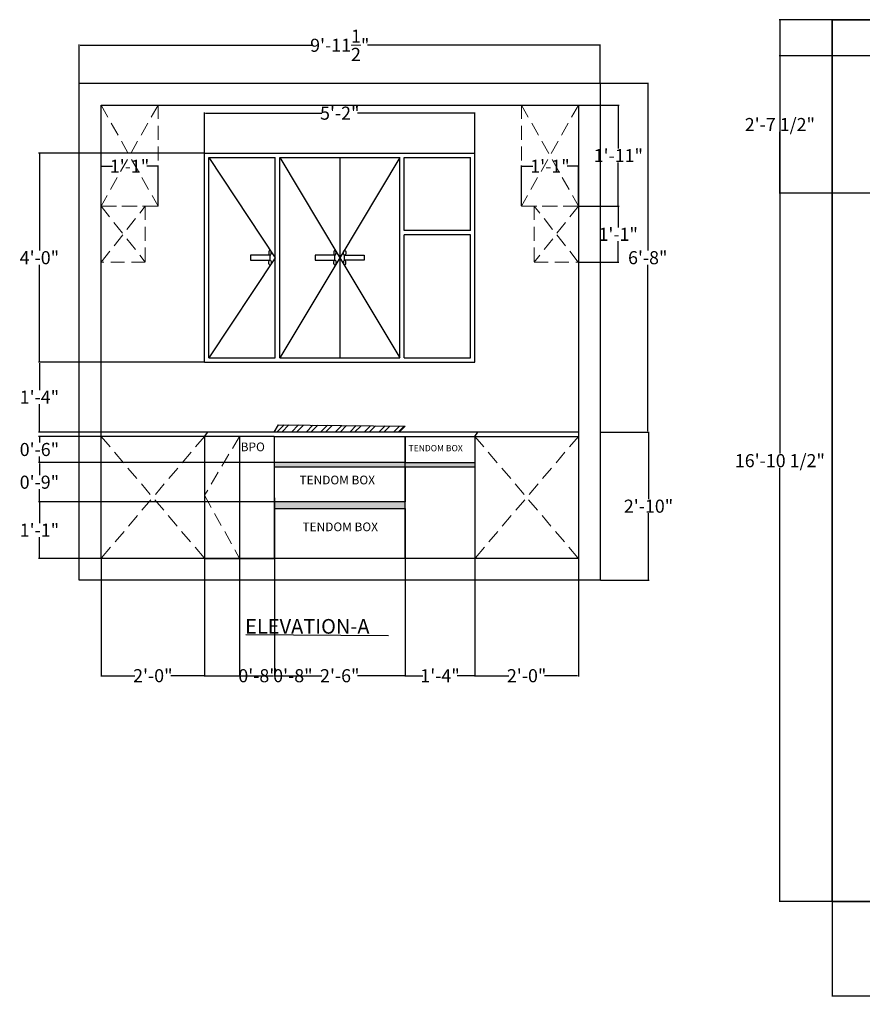
# Model space of a CAD drawing. Units: inches. Extents: x 1686244 to 1686928, y 1936095 to 1936489.
# Tile 1 of 11: x 1686285 to 1686478, y 1936095 to 1936321. Entities that reach past the tile are written whole.
import ezdxf

# ---------------------------------------------------------------- set-up
doc = ezdxf.new("R2010")
doc.units = ezdxf.units.IN
doc.header["$MEASUREMENT"] = 0
doc.linetypes.add('DASHED', pattern=[19.05, 12.7, -6.35])
for name, color, linetype, lineweight in [('A-ANNO-DIMS', 240, 'Continuous', 18), ('A-ANNO-TEXT', 7, 'Continuous', 18), ('A-CASE', 7, 'Continuous', 35), ('A-CASE-SWNG', 1, 'DASHED', 18), ('A-ELEV', 7, 'Continuous', 25), ('A-ELEV-PATT', 72, 'Continuous', 13)]:
    doc.layers.add(name, color=color, linetype=linetype, lineweight=lineweight)
doc.styles.get("Standard").update_dxf_attribs({"font": 'arial.ttf'})
doc.dimstyles.get("Standard").update_dxf_attribs({"dimtxt": 3, "dimasz": 0.18, "dimexe": 0.18, "dimexo": 0.0625, "dimgap": 0.09, "dimtad": 0, "dimtih": 1, "dimtoh": 1, "dimzin": 0, "dimdsep": 46, "dimlunit": 4, "dimtxsty": 'Standard', "dimcen": 0.09, "dimadec": 0, "dimazin": 0, "dimtfac": 1, "dimtofl": 0, "dimtmove": 0, "dimatfit": 3, "dimfxl": 1, "dimtolj": 1, "dimtzin": 0, "dimarcsym": 0})

# ---------------------------------------------------------------- blocks, each defined once
blk = doc.blocks.new('*D37')
at = {"layer": 'A-ANNO-DIMS', "color": 0, "lineweight": -2, "transparency": 16777216}
for p, q in [((1686298.55, 1936306.63), (1686298.55, 1936315.47)), ((1686298.73, 1936315.29), (1686351.96, 1936315.29)), ((1686417.87, 1936315.29), (1686364.63, 1936315.29)), ((1686418.05, 1936306.63), (1686418.05, 1936315.47))]:
    blk.add_line(p, q, dxfattribs=at)
at = {"layer": 'A-ANNO-DIMS', "color": 0, "transparency": 16777216}
for points in [[(1686298.73, 1936315.32), (1686298.73, 1936315.26), (1686298.55, 1936315.29)], [(1686417.87, 1936315.32), (1686417.87, 1936315.26), (1686418.05, 1936315.29)]]:
    blk.add_solid(points, dxfattribs=at)
at = {"layer": 'Defpoints', "color": 0, "transparency": 16777216}
for p in [(1686418.05, 1936315.29), (1686298.55, 1936306.57), (1686418.05, 1936306.57)]:
    blk.add_point(p, dxfattribs=at)
at = {"layer": 'A-ANNO-DIMS', "color": 0, "transparency": 16777216, "insert": (1686358.3, 1936315.29), "char_height": 3, "attachment_point": 5}
blk.add_mtext('\\A1;9\'-11{\\H1x;\\S1/2;}"', dxfattribs=at)
blk = doc.blocks.new('*D38')
at = {"layer": 'A-ANNO-DIMS', "color": 0, "lineweight": -2, "transparency": 16777216}
for p, q in [((1686418.11, 1936306.57), (1686429.13, 1936306.57)), ((1686428.95, 1936306.39), (1686428.95, 1936268.19)), ((1686428.95, 1936226.75), (1686428.95, 1936264.95)), ((1686418.11, 1936226.57), (1686429.13, 1936226.57))]:
    blk.add_line(p, q, dxfattribs=at)
at = {"layer": 'A-ANNO-DIMS', "color": 0, "transparency": 16777216}
for points in [[(1686428.92, 1936306.39), (1686428.98, 1936306.39), (1686428.95, 1936306.57)], [(1686428.92, 1936226.75), (1686428.98, 1936226.75), (1686428.95, 1936226.57)]]:
    blk.add_solid(points, dxfattribs=at)
at = {"layer": 'Defpoints', "color": 0, "transparency": 16777216}
for p in [(1686418.05, 1936306.57), (1686418.05, 1936226.57), (1686428.95, 1936226.57)]:
    blk.add_point(p, dxfattribs=at)
at = {"layer": 'A-ANNO-DIMS', "color": 0, "transparency": 16777216, "insert": (1686428.95, 1936266.57), "char_height": 3, "attachment_point": 5}
blk.add_mtext('\\A1;6\'-8"', dxfattribs=at)
blk = doc.blocks.new('*D39')
at = {"layer": 'A-ANNO-DIMS', "color": 0, "lineweight": -2, "transparency": 16777216}
for p, q in [((1686418.11, 1936226.57), (1686429.31, 1936226.57)), ((1686429.13, 1936226.39), (1686429.13, 1936211.19)), ((1686429.13, 1936192.75), (1686429.13, 1936207.95)), ((1686418.11, 1936192.57), (1686429.31, 1936192.57))]:
    blk.add_line(p, q, dxfattribs=at)
at = {"layer": 'A-ANNO-DIMS', "color": 0, "transparency": 16777216}
for points in [[(1686429.1, 1936226.39), (1686429.16, 1936226.39), (1686429.13, 1936226.57)], [(1686429.1, 1936192.75), (1686429.16, 1936192.75), (1686429.13, 1936192.57)]]:
    blk.add_solid(points, dxfattribs=at)
at = {"layer": 'Defpoints', "color": 0, "transparency": 16777216}
for p in [(1686418.05, 1936226.57), (1686418.05, 1936192.57), (1686429.13, 1936192.57)]:
    blk.add_point(p, dxfattribs=at)
at = {"layer": 'A-ANNO-DIMS', "color": 0, "transparency": 16777216, "insert": (1686429.13, 1936209.57), "char_height": 3, "attachment_point": 5}
blk.add_mtext('\\A1;2\'-10"', dxfattribs=at)
blk = doc.blocks.new('*D71')
at = {"layer": 'A-ANNO-DIMS', "color": 0, "lineweight": -2, "transparency": 16777216}
for p, q in [((1686303.55, 1936278.46), (1686303.55, 1936287.72)), ((1686303.73, 1936287.54), (1686306.14, 1936287.54)), ((1686316.43, 1936287.54), (1686314.01, 1936287.54)), ((1686316.61, 1936278.46), (1686316.61, 1936287.72))]:
    blk.add_line(p, q, dxfattribs=at)
at = {"layer": 'A-ANNO-DIMS', "color": 0, "transparency": 16777216}
for points in [[(1686303.73, 1936287.57), (1686303.73, 1936287.51), (1686303.55, 1936287.54)], [(1686316.43, 1936287.57), (1686316.43, 1936287.51), (1686316.61, 1936287.54)]]:
    blk.add_solid(points, dxfattribs=at)
at = {"layer": 'Defpoints', "color": 0, "transparency": 16777216}
for p in [(1686316.61, 1936287.54), (1686303.55, 1936278.39), (1686316.61, 1936278.39)]:
    blk.add_point(p, dxfattribs=at)
at = {"layer": 'A-ANNO-DIMS', "color": 0, "transparency": 16777216, "insert": (1686310.08, 1936287.54), "char_height": 3, "attachment_point": 5}
blk.add_mtext('\\A1;1\'-1"', dxfattribs=at)
blk = doc.blocks.new('*D72')
at = {"layer": 'A-ANNO-DIMS', "color": 0, "lineweight": -2, "transparency": 16777216}
for p, q in [((1686327.3, 1936290.63), (1686327.3, 1936299.9)), ((1686327.48, 1936299.72), (1686354.22, 1936299.72)), ((1686389.12, 1936299.72), (1686362.37, 1936299.72)), ((1686389.3, 1936290.63), (1686389.3, 1936299.9))]:
    blk.add_line(p, q, dxfattribs=at)
at = {"layer": 'A-ANNO-DIMS', "color": 0, "transparency": 16777216}
for points in [[(1686327.48, 1936299.75), (1686327.48, 1936299.69), (1686327.3, 1936299.72)], [(1686389.12, 1936299.75), (1686389.12, 1936299.69), (1686389.3, 1936299.72)]]:
    blk.add_solid(points, dxfattribs=at)
at = {"layer": 'Defpoints', "color": 0, "transparency": 16777216}
for p in [(1686389.3, 1936299.72), (1686327.3, 1936290.57), (1686389.3, 1936290.57)]:
    blk.add_point(p, dxfattribs=at)
at = {"layer": 'A-ANNO-DIMS', "color": 0, "transparency": 16777216, "insert": (1686358.3, 1936299.72), "char_height": 3, "attachment_point": 5}
blk.add_mtext('\\A1;5\'-2"', dxfattribs=at)
blk = doc.blocks.new('*D73')
at = {"layer": 'A-ANNO-DIMS', "color": 0, "lineweight": -2, "transparency": 16777216}
for p, q in [((1686399.99, 1936278.46), (1686399.99, 1936287.72)), ((1686400.17, 1936287.54), (1686402.58, 1936287.54)), ((1686412.87, 1936287.54), (1686410.45, 1936287.54)), ((1686413.05, 1936278.46), (1686413.05, 1936287.72))]:
    blk.add_line(p, q, dxfattribs=at)
at = {"layer": 'A-ANNO-DIMS', "color": 0, "transparency": 16777216}
for points in [[(1686400.17, 1936287.57), (1686400.17, 1936287.51), (1686399.99, 1936287.54)], [(1686412.87, 1936287.57), (1686412.87, 1936287.51), (1686413.05, 1936287.54)]]:
    blk.add_solid(points, dxfattribs=at)
at = {"layer": 'Defpoints', "color": 0, "transparency": 16777216}
for p in [(1686413.05, 1936287.54), (1686399.99, 1936278.39), (1686413.05, 1936278.39)]:
    blk.add_point(p, dxfattribs=at)
at = {"layer": 'A-ANNO-DIMS', "color": 0, "transparency": 16777216, "insert": (1686406.52, 1936287.54), "char_height": 3, "attachment_point": 5}
blk.add_mtext('\\A1;1\'-1"', dxfattribs=at)
blk = doc.blocks.new('*D74')
at = {"layer": 'A-ANNO-DIMS', "color": 0, "lineweight": -2, "transparency": 16777216}
for p, q in [((1686413.11, 1936301.57), (1686422.38, 1936301.57)), ((1686422.2, 1936301.39), (1686422.2, 1936291.58)), ((1686422.2, 1936278.57), (1686422.2, 1936288.38)), ((1686413.11, 1936278.39), (1686422.38, 1936278.39))]:
    blk.add_line(p, q, dxfattribs=at)
at = {"layer": 'A-ANNO-DIMS', "color": 0, "transparency": 16777216}
for points in [[(1686422.17, 1936301.39), (1686422.23, 1936301.39), (1686422.2, 1936301.57)], [(1686422.17, 1936278.57), (1686422.23, 1936278.57), (1686422.2, 1936278.39)]]:
    blk.add_solid(points, dxfattribs=at)
at = {"layer": 'Defpoints', "color": 0, "transparency": 16777216}
for p in [(1686413.05, 1936301.57), (1686413.05, 1936278.39), (1686422.2, 1936278.39)]:
    blk.add_point(p, dxfattribs=at)
at = {"layer": 'A-ANNO-DIMS', "color": 0, "transparency": 16777216, "insert": (1686422.2, 1936289.98), "char_height": 3, "attachment_point": 5}
blk.add_mtext('\\A1;1\'-11"', dxfattribs=at)
blk = doc.blocks.new('*D75')
at = {"layer": 'A-ANNO-DIMS', "color": 0, "lineweight": -2, "transparency": 16777216}
for p, q in [((1686413.11, 1936278.39), (1686422.38, 1936278.36)), ((1686422.2, 1936278.18), (1686422.18, 1936273.53)), ((1686422.15, 1936265.69), (1686422.17, 1936270.34)), ((1686413.06, 1936265.54), (1686422.33, 1936265.51))]:
    blk.add_line(p, q, dxfattribs=at)
at = {"layer": 'A-ANNO-DIMS', "color": 0, "transparency": 16777216}
for points in [[(1686422.17, 1936278.18), (1686422.23, 1936278.18), (1686422.2, 1936278.36)], [(1686422.12, 1936265.69), (1686422.18, 1936265.69), (1686422.15, 1936265.51)]]:
    blk.add_solid(points, dxfattribs=at)
at = {"layer": 'Defpoints', "color": 0, "transparency": 16777216}
for p in [(1686413.05, 1936278.39), (1686413, 1936265.54), (1686422.15, 1936265.51)]:
    blk.add_point(p, dxfattribs=at)
at = {"layer": 'A-ANNO-DIMS', "color": 0, "transparency": 16777216, "insert": (1686422.17, 1936271.93), "char_height": 3, "attachment_point": 5}
blk.add_mtext('\\A1;1\'-1"', dxfattribs=at)
blk = doc.blocks.new('*D76')
at = {"layer": 'A-ANNO-DIMS', "color": 0, "lineweight": -2, "transparency": 16777216}
for p, q in [((1686327.23, 1936290.57), (1686289.22, 1936290.57)), ((1686289.4, 1936290.39), (1686289.4, 1936268.19)), ((1686289.4, 1936242.75), (1686289.4, 1936264.95)), ((1686327.23, 1936242.57), (1686289.22, 1936242.57))]:
    blk.add_line(p, q, dxfattribs=at)
at = {"layer": 'A-ANNO-DIMS', "color": 0, "transparency": 16777216}
for points in [[(1686289.37, 1936290.39), (1686289.43, 1936290.39), (1686289.4, 1936290.57)], [(1686289.37, 1936242.75), (1686289.43, 1936242.75), (1686289.4, 1936242.57)]]:
    blk.add_solid(points, dxfattribs=at)
at = {"layer": 'Defpoints', "color": 0, "transparency": 16777216}
for p in [(1686327.3, 1936290.57), (1686289.4, 1936242.57), (1686327.3, 1936242.57)]:
    blk.add_point(p, dxfattribs=at)
at = {"layer": 'A-ANNO-DIMS', "color": 0, "transparency": 16777216, "insert": (1686289.4, 1936266.57), "char_height": 3, "attachment_point": 5}
blk.add_mtext('\\A1;4\'-0"', dxfattribs=at)
blk = doc.blocks.new('*D77')
at = {"layer": 'A-ANNO-DIMS', "color": 0, "lineweight": -2, "transparency": 16777216}
for p, q in [((1686327.23, 1936242.57), (1686289.22, 1936242.57)), ((1686289.4, 1936242.39), (1686289.4, 1936236.16)), ((1686289.4, 1936226.75), (1686289.4, 1936232.97)), ((1686303.48, 1936226.57), (1686289.22, 1936226.57))]:
    blk.add_line(p, q, dxfattribs=at)
at = {"layer": 'A-ANNO-DIMS', "color": 0, "transparency": 16777216}
for points in [[(1686289.37, 1936242.39), (1686289.43, 1936242.39), (1686289.4, 1936242.57)], [(1686289.37, 1936226.75), (1686289.43, 1936226.75), (1686289.4, 1936226.57)]]:
    blk.add_solid(points, dxfattribs=at)
at = {"layer": 'Defpoints', "color": 0, "transparency": 16777216}
for p in [(1686327.3, 1936242.57), (1686289.4, 1936226.57), (1686303.55, 1936226.57)]:
    blk.add_point(p, dxfattribs=at)
at = {"layer": 'A-ANNO-DIMS', "color": 0, "transparency": 16777216, "insert": (1686289.4, 1936234.57), "char_height": 3, "attachment_point": 5}
blk.add_mtext('\\A1;1\'-4"', dxfattribs=at)
blk = doc.blocks.new('*D78')
at = {"layer": 'A-ANNO-DIMS', "color": 0, "lineweight": -2, "transparency": 16777216}
for p, q in [((1686343.22, 1936225.57), (1686289.22, 1936225.57)), ((1686289.4, 1936225.39), (1686289.4, 1936224.19)), ((1686289.4, 1936219.75), (1686289.4, 1936220.95)), ((1686343.23, 1936219.57), (1686289.22, 1936219.57))]:
    blk.add_line(p, q, dxfattribs=at)
at = {"layer": 'A-ANNO-DIMS', "color": 0, "transparency": 16777216}
for points in [[(1686289.37, 1936225.39), (1686289.43, 1936225.39), (1686289.4, 1936225.57)], [(1686289.37, 1936219.75), (1686289.43, 1936219.75), (1686289.4, 1936219.57)]]:
    blk.add_solid(points, dxfattribs=at)
at = {"layer": 'Defpoints', "color": 0, "transparency": 16777216}
for p in [(1686343.28, 1936225.57), (1686289.4, 1936219.57), (1686343.3, 1936219.57)]:
    blk.add_point(p, dxfattribs=at)
at = {"layer": 'A-ANNO-DIMS', "color": 0, "transparency": 16777216, "insert": (1686289.4, 1936222.57), "char_height": 3, "attachment_point": 5}
blk.add_mtext('\\A1;0\'-6"', dxfattribs=at)
blk = doc.blocks.new('*D79')
at = {"layer": 'A-ANNO-DIMS', "color": 0, "lineweight": -2, "transparency": 16777216}
for p, q in [((1686343.23, 1936219.57), (1686289.22, 1936219.57)), ((1686289.4, 1936219.39), (1686289.4, 1936216.69)), ((1686289.4, 1936210.75), (1686289.4, 1936213.45)), ((1686343.23, 1936210.57), (1686289.22, 1936210.57))]:
    blk.add_line(p, q, dxfattribs=at)
at = {"layer": 'A-ANNO-DIMS', "color": 0, "transparency": 16777216}
for points in [[(1686289.37, 1936219.39), (1686289.43, 1936219.39), (1686289.4, 1936219.57)], [(1686289.37, 1936210.75), (1686289.43, 1936210.75), (1686289.4, 1936210.57)]]:
    blk.add_solid(points, dxfattribs=at)
at = {"layer": 'Defpoints', "color": 0, "transparency": 16777216}
for p in [(1686343.3, 1936219.57), (1686289.4, 1936210.57), (1686343.3, 1936210.57)]:
    blk.add_point(p, dxfattribs=at)
at = {"layer": 'A-ANNO-DIMS', "color": 0, "transparency": 16777216, "insert": (1686289.4, 1936215.07), "char_height": 3, "attachment_point": 5}
blk.add_mtext('\\A1;0\'-9"', dxfattribs=at)
blk = doc.blocks.new('*D80')
at = {"layer": 'A-ANNO-DIMS', "color": 0, "lineweight": -2, "transparency": 16777216}
for p, q in [((1686343.23, 1936210.57), (1686289.22, 1936210.57)), ((1686289.4, 1936210.39), (1686289.4, 1936205.66)), ((1686289.4, 1936197.75), (1686289.4, 1936202.47)), ((1686343.23, 1936197.57), (1686289.22, 1936197.57))]:
    blk.add_line(p, q, dxfattribs=at)
at = {"layer": 'A-ANNO-DIMS', "color": 0, "transparency": 16777216}
for points in [[(1686289.37, 1936210.39), (1686289.43, 1936210.39), (1686289.4, 1936210.57)], [(1686289.37, 1936197.75), (1686289.43, 1936197.75), (1686289.4, 1936197.57)]]:
    blk.add_solid(points, dxfattribs=at)
at = {"layer": 'Defpoints', "color": 0, "transparency": 16777216}
for p in [(1686343.3, 1936210.57), (1686289.4, 1936197.57), (1686343.3, 1936197.57)]:
    blk.add_point(p, dxfattribs=at)
at = {"layer": 'A-ANNO-DIMS', "color": 0, "transparency": 16777216, "insert": (1686289.4, 1936204.07), "char_height": 3, "attachment_point": 5}
blk.add_mtext('\\A1;1\'-1"', dxfattribs=at)
blk = doc.blocks.new('*D81')
at = {"layer": 'A-ANNO-DIMS', "color": 0, "lineweight": -2, "transparency": 16777216}
for p, q in [((1686303.55, 1936197.51), (1686303.55, 1936170.5)), ((1686327.3, 1936197.51), (1686327.3, 1936170.5)), ((1686303.73, 1936170.68), (1686311.32, 1936170.68)), ((1686327.12, 1936170.68), (1686319.53, 1936170.68))]:
    blk.add_line(p, q, dxfattribs=at)
at = {"layer": 'A-ANNO-DIMS', "color": 0, "transparency": 16777216}
for points in [[(1686303.73, 1936170.71), (1686303.73, 1936170.65), (1686303.55, 1936170.68)], [(1686327.12, 1936170.71), (1686327.12, 1936170.65), (1686327.3, 1936170.68)]]:
    blk.add_solid(points, dxfattribs=at)
at = {"layer": 'Defpoints', "color": 0, "transparency": 16777216}
for p in [(1686303.55, 1936197.57), (1686327.3, 1936197.57), (1686327.3, 1936170.68)]:
    blk.add_point(p, dxfattribs=at)
at = {"layer": 'A-ANNO-DIMS', "color": 0, "transparency": 16777216, "insert": (1686315.42, 1936170.68), "char_height": 3, "attachment_point": 5}
blk.add_mtext('\\A1;2\'-0"', dxfattribs=at)
blk = doc.blocks.new('*D82')
at = {"layer": 'A-ANNO-DIMS', "color": 0, "lineweight": -2, "transparency": 16777216}
for p, q in [((1686327.3, 1936197.51), (1686327.3, 1936170.5)), ((1686335.3, 1936197.51), (1686335.3, 1936170.5)), ((1686327.48, 1936170.68), (1686335.12, 1936170.68)), ((1686335.3, 1936170.68), (1686335.48, 1936170.68))]:
    blk.add_line(p, q, dxfattribs=at)
at = {"layer": 'A-ANNO-DIMS', "color": 0, "transparency": 16777216}
for points in [[(1686327.48, 1936170.71), (1686327.48, 1936170.65), (1686327.3, 1936170.68)], [(1686335.12, 1936170.71), (1686335.12, 1936170.65), (1686335.3, 1936170.68)]]:
    blk.add_solid(points, dxfattribs=at)
at = {"layer": 'Defpoints', "color": 0, "transparency": 16777216}
for p in [(1686327.3, 1936197.57), (1686335.3, 1936197.57), (1686335.3, 1936170.68)]:
    blk.add_point(p, dxfattribs=at)
at = {"layer": 'A-ANNO-DIMS', "color": 0, "transparency": 16777216, "insert": (1686339.55, 1936170.68), "char_height": 3, "attachment_point": 5}
blk.add_mtext('\\A1;0\'-8"', dxfattribs=at)
blk = doc.blocks.new('*D83')
at = {"layer": 'A-ANNO-DIMS', "color": 0, "lineweight": -2, "transparency": 16777216}
for p, q in [((1686335.3, 1936197.51), (1686335.3, 1936170.5)), ((1686343.3, 1936197.51), (1686343.3, 1936170.5)), ((1686335.48, 1936170.68), (1686343.12, 1936170.68)), ((1686343.3, 1936170.68), (1686343.48, 1936170.68))]:
    blk.add_line(p, q, dxfattribs=at)
at = {"layer": 'A-ANNO-DIMS', "color": 0, "transparency": 16777216}
for points in [[(1686335.48, 1936170.71), (1686335.48, 1936170.65), (1686335.3, 1936170.68)], [(1686343.12, 1936170.71), (1686343.12, 1936170.65), (1686343.3, 1936170.68)]]:
    blk.add_solid(points, dxfattribs=at)
at = {"layer": 'Defpoints', "color": 0, "transparency": 16777216}
for p in [(1686335.3, 1936197.57), (1686343.3, 1936197.57), (1686343.3, 1936170.68)]:
    blk.add_point(p, dxfattribs=at)
at = {"layer": 'A-ANNO-DIMS', "color": 0, "transparency": 16777216, "insert": (1686347.55, 1936170.68), "char_height": 3, "attachment_point": 5}
blk.add_mtext('\\A1;0\'-8"', dxfattribs=at)
blk = doc.blocks.new('*D84')
at = {"layer": 'A-ANNO-DIMS', "color": 0, "lineweight": -2, "transparency": 16777216}
for p, q in [((1686343.3, 1936197.51), (1686343.3, 1936170.5)), ((1686373.3, 1936197.51), (1686373.3, 1936170.5)), ((1686343.48, 1936170.68), (1686354.19, 1936170.68)), ((1686373.12, 1936170.68), (1686362.4, 1936170.68))]:
    blk.add_line(p, q, dxfattribs=at)
at = {"layer": 'A-ANNO-DIMS', "color": 0, "transparency": 16777216}
for points in [[(1686343.48, 1936170.71), (1686343.48, 1936170.65), (1686343.3, 1936170.68)], [(1686373.12, 1936170.71), (1686373.12, 1936170.65), (1686373.3, 1936170.68)]]:
    blk.add_solid(points, dxfattribs=at)
at = {"layer": 'Defpoints', "color": 0, "transparency": 16777216}
for p in [(1686343.3, 1936197.57), (1686373.3, 1936197.57), (1686373.3, 1936170.68)]:
    blk.add_point(p, dxfattribs=at)
at = {"layer": 'A-ANNO-DIMS', "color": 0, "transparency": 16777216, "insert": (1686358.3, 1936170.68), "char_height": 3, "attachment_point": 5}
blk.add_mtext('\\A1;2\'-6"', dxfattribs=at)
blk = doc.blocks.new('*D85')
at = {"layer": 'A-ANNO-DIMS', "color": 0, "lineweight": -2, "transparency": 16777216}
for p, q in [((1686373.3, 1936197.51), (1686373.3, 1936170.5)), ((1686389.3, 1936197.51), (1686389.3, 1936170.5)), ((1686373.48, 1936170.68), (1686377.36, 1936170.68)), ((1686389.12, 1936170.68), (1686385.23, 1936170.68))]:
    blk.add_line(p, q, dxfattribs=at)
at = {"layer": 'A-ANNO-DIMS', "color": 0, "transparency": 16777216}
for points in [[(1686373.48, 1936170.71), (1686373.48, 1936170.65), (1686373.3, 1936170.68)], [(1686389.12, 1936170.71), (1686389.12, 1936170.65), (1686389.3, 1936170.68)]]:
    blk.add_solid(points, dxfattribs=at)
at = {"layer": 'Defpoints', "color": 0, "transparency": 16777216}
for p in [(1686373.3, 1936197.57), (1686389.3, 1936197.57), (1686389.3, 1936170.68)]:
    blk.add_point(p, dxfattribs=at)
at = {"layer": 'A-ANNO-DIMS', "color": 0, "transparency": 16777216, "insert": (1686381.3, 1936170.68), "char_height": 3, "attachment_point": 5}
blk.add_mtext('\\A1;1\'-4"', dxfattribs=at)
blk = doc.blocks.new('*D86')
at = {"layer": 'A-ANNO-DIMS', "color": 0, "lineweight": -2, "transparency": 16777216}
for p, q in [((1686389.3, 1936197.51), (1686389.3, 1936170.5)), ((1686413.05, 1936197.51), (1686413.05, 1936170.5)), ((1686389.48, 1936170.68), (1686397.07, 1936170.68)), ((1686412.87, 1936170.68), (1686405.28, 1936170.68))]:
    blk.add_line(p, q, dxfattribs=at)
at = {"layer": 'A-ANNO-DIMS', "color": 0, "transparency": 16777216}
for points in [[(1686389.48, 1936170.71), (1686389.48, 1936170.65), (1686389.3, 1936170.68)], [(1686412.87, 1936170.71), (1686412.87, 1936170.65), (1686413.05, 1936170.68)]]:
    blk.add_solid(points, dxfattribs=at)
at = {"layer": 'Defpoints', "color": 0, "transparency": 16777216}
for p in [(1686389.3, 1936197.57), (1686413.05, 1936197.57), (1686413.05, 1936170.68)]:
    blk.add_point(p, dxfattribs=at)
at = {"layer": 'A-ANNO-DIMS', "color": 0, "transparency": 16777216, "insert": (1686401.17, 1936170.68), "char_height": 3, "attachment_point": 5}
blk.add_mtext('\\A1;2\'-0"', dxfattribs=at)
blk = doc.blocks.new('*D113')
at = {"layer": 'A-ANNO-DIMS', "color": 0, "lineweight": -2, "transparency": 16777216}
for p, q in [((1686471.29, 1936118.8), (1686471.29, 1936097.09)), ((1686608.35, 1936118.8), (1686608.35, 1936097.09)), ((1686471.47, 1936097.27), (1686534.72, 1936097.27)), ((1686608.17, 1936097.27), (1686544.92, 1936097.27))]:
    blk.add_line(p, q, dxfattribs=at)
at = {"layer": 'A-ANNO-DIMS', "color": 0, "transparency": 16777216}
for points in [[(1686471.47, 1936097.3), (1686471.47, 1936097.24), (1686471.29, 1936097.27)], [(1686608.17, 1936097.3), (1686608.17, 1936097.24), (1686608.35, 1936097.27)]]:
    blk.add_solid(points, dxfattribs=at)
at = {"layer": 'Defpoints', "color": 0, "transparency": 16777216}
for p in [(1686471.29, 1936118.86), (1686608.35, 1936118.86), (1686608.35, 1936097.27)]:
    blk.add_point(p, dxfattribs=at)
at = {"layer": 'A-ANNO-DIMS', "color": 0, "transparency": 16777216, "insert": (1686539.82, 1936097.27), "char_height": 3, "attachment_point": 5}
blk.add_mtext('\\A1;11\'-5"', dxfattribs=at)
blk = doc.blocks.new('*D114')
at = {"layer": 'A-ANNO-DIMS', "color": 0, "lineweight": -2, "transparency": 16777216}
for p, q in [((1686471.23, 1936321.16), (1686459.08, 1936321.16)), ((1686459.26, 1936320.98), (1686459.26, 1936221.65)), ((1686459.26, 1936119.04), (1686459.26, 1936218.37)), ((1686471.23, 1936118.86), (1686459.08, 1936118.86))]:
    blk.add_line(p, q, dxfattribs=at)
at = {"layer": 'A-ANNO-DIMS', "color": 0, "transparency": 16777216}
for points in [[(1686459.23, 1936320.98), (1686459.29, 1936320.98), (1686459.26, 1936321.16)], [(1686459.23, 1936119.04), (1686459.29, 1936119.04), (1686459.26, 1936118.86)]]:
    blk.add_solid(points, dxfattribs=at)
at = {"layer": 'Defpoints', "color": 0, "transparency": 16777216}
for p in [(1686459.26, 1936321.16), (1686471.29, 1936321.16), (1686471.29, 1936118.86)]:
    blk.add_point(p, dxfattribs=at)
at = {"layer": 'A-ANNO-DIMS', "color": 0, "transparency": 16777216, "insert": (1686459.26, 1936220.01), "char_height": 3, "attachment_point": 5}
blk.add_mtext('\\A1;16\'-10 1/2"', dxfattribs=at)
blk = doc.blocks.new('*D122')
at = {"layer": 'A-ANNO-DIMS', "color": 0, "lineweight": -2, "transparency": 16777216}
for p, q in [((1686504.4, 1936312.86), (1686459.08, 1936312.86)), ((1686459.26, 1936312.68), (1686459.26, 1936298.75)), ((1686459.26, 1936281.54), (1686459.26, 1936295.47)), ((1686504.4, 1936281.36), (1686459.08, 1936281.36))]:
    blk.add_line(p, q, dxfattribs=at)
at = {"layer": 'A-ANNO-DIMS', "color": 0, "transparency": 16777216}
for points in [[(1686459.23, 1936312.68), (1686459.29, 1936312.68), (1686459.26, 1936312.86)], [(1686459.23, 1936281.54), (1686459.29, 1936281.54), (1686459.26, 1936281.36)]]:
    blk.add_solid(points, dxfattribs=at)
at = {"layer": 'Defpoints', "color": 0, "transparency": 16777216}
for p in [(1686504.46, 1936312.86), (1686459.26, 1936281.36), (1686504.46, 1936281.36)]:
    blk.add_point(p, dxfattribs=at)
at = {"layer": 'A-ANNO-DIMS', "color": 0, "transparency": 16777216, "insert": (1686459.26, 1936297.11), "char_height": 3, "attachment_point": 5}
blk.add_mtext('\\A1;2\'-7 1/2"', dxfattribs=at)

msp = doc.modelspace()

# ---------------------------------------------------------------- hatches: boundary and pattern name
at = {"layer": 'A-ELEV-PATT'}
h = msp.add_hatch(dxfattribs=at)
h.set_pattern_fill('ANSI32', color=256, scale=6.3)
h.paths.add_polyline_path([(1686373.297, 1936227.92), (1686344.245, 1936228.245), (1686343.282, 1936226.568), (1686371.953, 1936226.568)])
h = msp.add_hatch(color=256, dxfattribs=at)
h.dxf.hatch_style = 1
h.paths.add_polyline_path([(1686373.297, 1936219.568), (1686343.297, 1936219.568), (1686343.297, 1936218.568), (1686373.297, 1936218.568)])
h = msp.add_hatch(color=256, dxfattribs=at)
h.dxf.hatch_style = 1
h.paths.add_polyline_path([(1686389.297, 1936219.568), (1686373.297, 1936219.568), (1686373.297, 1936218.568), (1686389.297, 1936218.568)])
h = msp.add_hatch(color=256, dxfattribs=at)
h.dxf.hatch_style = 1
h.paths.add_polyline_path([(1686373.297, 1936210.568), (1686343.297, 1936210.568), (1686343.298, 1936209.068), (1686373.297, 1936209.068)])

# ---------------------------------------------------------------- linework, layer by layer
at = {"layer": 'A-CASE'}
msp.add_line((1686471.291, 1936321.159), (1686480.291, 1936321.159), dxfattribs=at)
msp.add_lwpolyline([(1686608.345, 1936303.497), (1686608.345, 1936118.864), (1686471.291, 1936118.864), (1686471.291, 1936321.159)], dxfattribs=at)
at = {"layer": 'A-CASE-SWNG', "ltscale": 0.25}
for p, q in [((1686316.608, 1936301.568), (1686303.547, 1936278.393)), ((1686303.547, 1936301.568), (1686316.608, 1936278.393)), ((1686399.986, 1936301.568), (1686413.047, 1936278.393)), ((1686413.047, 1936301.568), (1686399.986, 1936278.393)), ((1686327.297, 1936225.568), (1686303.547, 1936197.568)), ((1686303.547, 1936225.568), (1686327.297, 1936197.568)), ((1686335.297, 1936225.568), (1686327.297, 1936212.068)), ((1686413.047, 1936225.568), (1686389.297, 1936197.568)), ((1686389.297, 1936225.568), (1686413.047, 1936197.568)), ((1686327.297, 1936212.068), (1686335.297, 1936197.568))]:
    msp.add_line(p, q, dxfattribs=at)
for points in [[(1686303.547, 1936301.568), (1686316.608, 1936301.568), (1686316.608, 1936278.393), (1686303.547, 1936278.393), (1686313.697, 1936278.393), (1686313.697, 1936265.542), (1686303.593, 1936265.542), (1686313.697, 1936278.393)], [(1686413.047, 1936301.568), (1686399.986, 1936301.568), (1686399.986, 1936278.393), (1686413.047, 1936278.393), (1686402.897, 1936278.393), (1686402.897, 1936265.542), (1686413.001, 1936265.542), (1686402.897, 1936278.393)], [(1686303.547, 1936278.393), (1686313.697, 1936265.542)], [(1686413.047, 1936278.393), (1686402.897, 1936265.542)]]:
    msp.add_lwpolyline(points, dxfattribs=at)
at = {"layer": 'A-ELEV'}
for p, q in [((1686327.297, 1936242.568), (1686327.297, 1936290.568)), ((1686327.297, 1936290.568), (1686389.297, 1936290.568)), ((1686389.297, 1936242.568), (1686389.297, 1936290.568)), ((1686328.297, 1936243.568), (1686328.297, 1936289.568)), ((1686328.297, 1936289.568), (1686343.517, 1936289.568)), ((1686328.297, 1936289.568), (1686343.517, 1936266.568)), ((1686343.517, 1936243.568), (1686343.517, 1936289.568)), ((1686344.517, 1936243.568), (1686344.517, 1936289.568)), ((1686344.517, 1936289.568), (1686372.078, 1936289.568)), ((1686344.517, 1936289.568), (1686358.297, 1936266.568)), ((1686358.297, 1936289.568), (1686358.297, 1936243.568)), ((1686372.078, 1936289.568), (1686358.297, 1936266.568)), ((1686372.078, 1936243.568), (1686372.078, 1936289.568)), ((1686373.078, 1936289.568), (1686388.297, 1936289.568)), ((1686373.078, 1936272.841), (1686373.078, 1936289.568)), ((1686388.297, 1936272.841), (1686388.297, 1936289.568)), ((1686388.297, 1936272.841), (1686373.078, 1936272.841)), ((1686373.078, 1936243.568), (1686373.078, 1936271.841)), ((1686388.297, 1936271.841), (1686373.078, 1936271.841)), ((1686388.297, 1936243.568), (1686388.297, 1936271.841)), ((1686343.517, 1936266.568), (1686328.297, 1936243.568)), ((1686358.297, 1936266.568), (1686344.517, 1936243.568)), ((1686358.297, 1936266.568), (1686372.078, 1936243.568)), ((1686327.297, 1936242.568), (1686389.297, 1936242.568)), ((1686328.297, 1936243.568), (1686343.517, 1936243.568)), ((1686344.517, 1936243.568), (1686372.078, 1936243.568)), ((1686373.078, 1936243.568), (1686388.297, 1936243.568)), ((1686327.297, 1936225.568), (1686328.048, 1936226.568)), ((1686343.282, 1936226.568), (1686344.245, 1936228.245)), ((1686344.245, 1936228.245), (1686373.297, 1936227.92)), ((1686373.297, 1936227.92), (1686371.953, 1936226.568)), ((1686389.297, 1936225.568), (1686389.985, 1936226.568)), ((1686343.283, 1936225.568), (1686303.547, 1936225.568)), ((1686327.297, 1936225.568), (1686327.297, 1936197.568)), ((1686335.297, 1936225.568), (1686335.297, 1936197.568)), ((1686343.283, 1936225.568), (1686343.309, 1936197.568)), ((1686343.297, 1936197.568), (1686343.297, 1936225.568)), ((1686373.297, 1936197.568), (1686373.297, 1936225.568)), ((1686373.297, 1936225.568), (1686413.047, 1936225.568)), ((1686389.297, 1936225.568), (1686389.297, 1936197.568)), ((1686373.297, 1936219.568), (1686389.297, 1936219.568)), ((1686373.297, 1936218.568), (1686389.297, 1936218.568)), ((1686327.297, 1936197.568), (1686343.297, 1936197.568)), ((1686389.297, 1936197.568), (1686373.297, 1936197.568)), ((1686369.453, 1936179.83), (1686336.733, 1936180.086))]:
    msp.add_line(p, q, dxfattribs=at)
for points in [[(1686298.547, 1936226.568), (1686298.547, 1936306.568), (1686418.047, 1936306.568), (1686418.047, 1936226.568)], [(1686303.547, 1936226.568), (1686303.547, 1936301.568), (1686413.047, 1936301.568), (1686413.047, 1936226.568)], [(1686418.047, 1936226.568), (1686418.047, 1936192.568), (1686298.547, 1936192.568), (1686298.547, 1936226.568)], [(1686413.047, 1936226.568), (1686413.047, 1936197.568), (1686303.547, 1936197.568), (1686303.547, 1936226.568)], [(1686413.047, 1936226.568), (1686303.547, 1936226.568)], [(1686343.297, 1936225.568), (1686373.297, 1936225.568), (1686373.297, 1936219.568), (1686343.297, 1936219.568), (1686343.297, 1936225.568)]]:
    msp.add_lwpolyline(points, dxfattribs=at)
for points in [[(1686342.299, 1936267.116), (1686337.802, 1936267.116), (1686337.802, 1936266.02), (1686342.299, 1936266.02)], [(1686357.175, 1936267.116), (1686352.678, 1936267.116), (1686352.678, 1936266.02), (1686357.175, 1936266.02)], [(1686359.419, 1936267.116), (1686363.916, 1936267.116), (1686363.916, 1936266.02), (1686359.419, 1936266.02)], [(1686343.297, 1936218.568), (1686373.297, 1936218.568), (1686373.297, 1936210.568), (1686343.297, 1936210.568)], [(1686343.297, 1936209.068), (1686373.297, 1936209.068), (1686373.297, 1936197.568), (1686343.297, 1936197.568)]]:
    msp.add_lwpolyline(points, close=True, dxfattribs=at)
at = {"layer": 'A-ELEV', "extrusion": (0, 0, -1)}
for centre, major_axis in [((1686342.299, 1936267.703), (0, 0.587)), ((1686357.175, 1936267.703), (0, 0.587)), ((1686359.419, 1936265.433), (0, -0.587))]:
    msp.add_ellipse(centre, major_axis=major_axis, ratio=0.4573838, dxfattribs=at)
at = {"layer": 'A-ELEV'}
for centre, major_axis in [((1686359.419, 1936267.703), (0, 0.587)), ((1686342.299, 1936265.433), (0, -0.587)), ((1686357.175, 1936265.433), (0, -0.587))]:
    msp.add_ellipse(centre, major_axis=major_axis, ratio=0.4573838, dxfattribs=at)

# ---------------------------------------------------------------- texts
at = {"layer": 'A-ANNO-TEXT'}
for s, height, p in [('BPO', 2, (1686335.573, 1936222.17)), ('TENDOM BOX', 1.4355, (1686374.078, 1936222.157)), ('TENDOM BOX', 2, (1686349.059, 1936214.573)), ('TENDOM BOX', 2, (1686349.748, 1936203.823)), ('ELEVATION-A', 3.36498, (1686336.594, 1936180.317))]:
    msp.add_text(s, height=height, dxfattribs=at).set_placement(p)

# ---------------------------------------------------------------- dimensions: what is measured, and where the dimension line sits
at = {"layer": 'A-ANNO-DIMS'}
for base, p1, p2, angle, override, picture, middle in [((1686459.261, 1936321.159), (1686471.291, 1936118.864), (1686471.291, 1936321.159), 90, {"dimdec": 1, "dimlfac": 1, "dimrnd": 0, "dimzin": 1, "dimdsep": 46, "dimlunit": 4, "dimfrac": 2}, '*D114', (1686459.261, 1936220.012)), ((1686459.261, 1936281.362), (1686504.458, 1936312.864), (1686504.458, 1936281.362), 90, {"dimdec": 1, "dimlfac": 1, "dimrnd": 0, "dimzin": 1, "dimdsep": 46, "dimlunit": 4, "dimfrac": 2}, '*D122', (1686459.261, 1936297.113)), ((1686428.953, 1936226.568), (1686418.047, 1936306.568), (1686418.047, 1936226.568), 90, {"dimclrd": 0, "dimclre": 0, "dimclrt": 0}, '*D38', (1686428.953, 1936266.568)), ((1686422.197, 1936278.393), (1686413.047, 1936301.568), (1686413.047, 1936278.393), 270, {"dimdec": 1, "dimlfac": 1, "dimrnd": 0, "dimzin": 1, "dimdsep": 46, "dimlunit": 4, "dimfrac": 2}, '*D74', (1686422.197, 1936289.98)), ((1686289.397, 1936242.568), (1686327.297, 1936290.568), (1686327.297, 1936242.568), 90, {"dimdec": 1, "dimlfac": 1, "dimrnd": 0, "dimzin": 1, "dimdsep": 46, "dimlunit": 4, "dimfrac": 2}, '*D76', (1686289.397, 1936266.568)), ((1686422.151, 1936265.509), (1686413.047, 1936278.393), (1686413.001, 1936265.542), 269.79472, {"dimdec": 1, "dimlfac": 1, "dimrnd": 0, "dimzin": 1, "dimdsep": 46, "dimlunit": 4, "dimfrac": 2}, '*D75', (1686422.174, 1936271.934)), ((1686289.397, 1936226.568), (1686327.297, 1936242.568), (1686303.547, 1936226.568), 90, {"dimdec": 1, "dimlfac": 1, "dimrnd": 0, "dimzin": 1, "dimdsep": 46, "dimlunit": 4, "dimfrac": 2}, '*D77', (1686289.397, 1936234.568)), ((1686429.133, 1936192.568), (1686418.047, 1936226.568), (1686418.047, 1936192.568), 90, {"dimclrd": 0, "dimclre": 0, "dimclrt": 0}, '*D39', (1686429.133, 1936209.568)), ((1686289.397, 1936219.568), (1686343.283, 1936225.568), (1686343.297, 1936219.568), 90, {"dimdec": 1, "dimlfac": 1, "dimrnd": 0, "dimzin": 1, "dimdsep": 46, "dimlunit": 4, "dimfrac": 2}, '*D78', (1686289.397, 1936222.568)), ((1686289.397, 1936210.568), (1686343.297, 1936219.568), (1686343.297, 1936210.568), 90, {"dimdec": 1, "dimlfac": 1, "dimrnd": 0, "dimzin": 1, "dimdsep": 46, "dimlunit": 4, "dimfrac": 2}, '*D79', (1686289.397, 1936215.068)), ((1686289.397, 1936197.568), (1686343.297, 1936210.568), (1686343.297, 1936197.568), 90, {"dimdec": 1, "dimlfac": 1, "dimrnd": 0, "dimzin": 1, "dimdsep": 46, "dimlunit": 4, "dimfrac": 2}, '*D80', (1686289.397, 1936204.068))]:
    dim = msp.add_linear_dim(base=base, p1=p1, p2=p2, angle=angle, dimstyle='Standard', override=override, dxfattribs=at)
    dim.commit()
    dim.dimension.update_dxf_attribs({"geometry": picture, "text_midpoint": middle})
for base, p1, p2, override, picture, middle in [((1686418.047, 1936315.287), (1686298.547, 1936306.568), (1686418.047, 1936306.568), {"dimclrd": 0, "dimclre": 0, "dimclrt": 0}, '*D37', (1686358.297, 1936315.287)), ((1686389.297, 1936299.718), (1686327.297, 1936290.568), (1686389.297, 1936290.568), {"dimdec": 1, "dimlfac": 1, "dimrnd": 0, "dimzin": 1, "dimdsep": 46, "dimlunit": 4, "dimfrac": 2}, '*D72', (1686358.297, 1936299.718)), ((1686316.608, 1936287.543), (1686303.547, 1936278.393), (1686316.608, 1936278.393), {"dimdec": 1, "dimlfac": 1, "dimrnd": 0, "dimzin": 1, "dimdsep": 46, "dimlunit": 4, "dimfrac": 2}, '*D71', (1686310.078, 1936287.543)), ((1686413.047, 1936287.543), (1686399.986, 1936278.393), (1686413.047, 1936278.393), {"dimdec": 1, "dimlfac": 1, "dimrnd": 0, "dimzin": 1, "dimdsep": 46, "dimlunit": 4, "dimfrac": 2}, '*D73', (1686406.517, 1936287.543)), ((1686327.297084, 1936170.68037), (1686303.547084, 1936197.568047), (1686327.297084, 1936197.568047), {"dimdec": 1, "dimlfac": 1, "dimrnd": 0, "dimzin": 1, "dimdsep": 46, "dimlunit": 4, "dimfrac": 2}, '*D81', (1686315.422084, 1936170.68037)), ((1686335.297, 1936170.68), (1686327.297, 1936197.568), (1686335.297, 1936197.568), {"dimdec": 1, "dimlfac": 1, "dimrnd": 0, "dimzin": 1, "dimdsep": 46, "dimlunit": 4, "dimfrac": 2}, '*D82', (1686339.554, 1936170.68)), ((1686343.297, 1936170.68), (1686335.297, 1936197.568), (1686343.297, 1936197.568), {"dimdec": 1, "dimlfac": 1, "dimrnd": 0, "dimzin": 1, "dimdsep": 46, "dimlunit": 4, "dimfrac": 2}, '*D83', (1686347.554, 1936170.68)), ((1686373.297, 1936170.68), (1686343.297, 1936197.568), (1686373.297, 1936197.568), {"dimdec": 1, "dimlfac": 1, "dimrnd": 0, "dimzin": 1, "dimdsep": 46, "dimlunit": 4, "dimfrac": 2}, '*D84', (1686358.297, 1936170.68)), ((1686389.297, 1936170.68), (1686373.297, 1936197.568), (1686389.297, 1936197.568), {"dimdec": 1, "dimlfac": 1, "dimrnd": 0, "dimzin": 1, "dimdsep": 46, "dimlunit": 4, "dimfrac": 2}, '*D85', (1686381.297, 1936170.68)), ((1686413.047084, 1936170.68037), (1686389.297084, 1936197.568047), (1686413.047084, 1936197.568047), {"dimdec": 1, "dimlfac": 1, "dimrnd": 0, "dimzin": 1, "dimdsep": 46, "dimlunit": 4, "dimfrac": 2}, '*D86', (1686401.172084, 1936170.68037)), ((1686608.345, 1936097.275), (1686471.291, 1936118.864), (1686608.345, 1936118.864), {"dimdec": 1, "dimlfac": 1, "dimrnd": 0, "dimzin": 1, "dimdsep": 46, "dimlunit": 4, "dimfrac": 2}, '*D113', (1686539.818, 1936097.275))]:
    dim = msp.add_linear_dim(base=base, p1=p1, p2=p2, dimstyle='Standard', override=override, dxfattribs=at)
    dim.commit()
    dim.dimension.update_dxf_attribs({"geometry": picture, "text_midpoint": middle})

doc.saveas('drawing.dxf')
